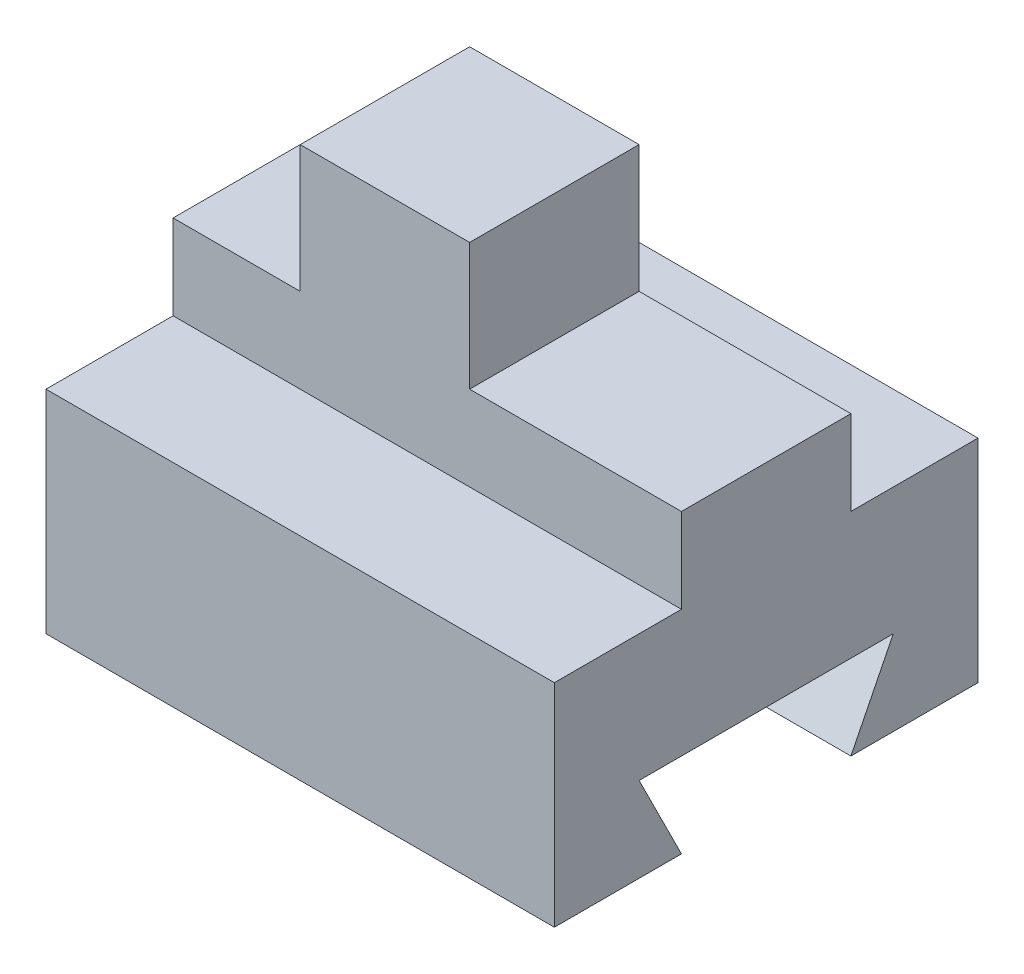
ISO-10303-21;
HEADER;
FILE_DESCRIPTION(('STEP AP214'),'2;1');
FILE_NAME('part.step','',(''),(''),'','','');
FILE_SCHEMA(('AUTOMOTIVE_DESIGN { 1 0 10303 214 1 1 1 1 }'));
ENDSEC;
DATA;
#1=APPLICATION_CONTEXT('core data for automotive mechanical design processes');
#2=APPLICATION_PROTOCOL_DEFINITION('international standard','automotive_design',2000,#1);
#3=PRODUCT_CONTEXT('',#1,'mechanical');
#4=PRODUCT('Part','Part','',(#3));
#5=PRODUCT_RELATED_PRODUCT_CATEGORY('part','',(#4));
#6=PRODUCT_DEFINITION_FORMATION('','',#4);
#7=PRODUCT_DEFINITION_CONTEXT('part definition',#1,'design');
#8=PRODUCT_DEFINITION('design','',#6,#7);
#9=PRODUCT_DEFINITION_SHAPE('','',#8);
#10=(LENGTH_UNIT() NAMED_UNIT(*) SI_UNIT(.MILLI.,.METRE.));
#11=(NAMED_UNIT(*) PLANE_ANGLE_UNIT() SI_UNIT($,.RADIAN.));
#12=(NAMED_UNIT(*) SI_UNIT($,.STERADIAN.) SOLID_ANGLE_UNIT());
#13=UNCERTAINTY_MEASURE_WITH_UNIT(LENGTH_MEASURE(1.E-05),#10,'distance_accuracy_value','');
#14=(GEOMETRIC_REPRESENTATION_CONTEXT(3) GLOBAL_UNCERTAINTY_ASSIGNED_CONTEXT((#13)) GLOBAL_UNIT_ASSIGNED_CONTEXT((#10,
#11,#12)) REPRESENTATION_CONTEXT('',''));
#15=CARTESIAN_POINT('',(0.,0.,0.));
#16=DIRECTION('',(0.,0.,1.));
#17=DIRECTION('',(1.,0.,0.));
#18=AXIS2_PLACEMENT_3D('',#15,#16,#17);
#19=CARTESIAN_POINT('',(30.,0.,25.));
#20=DIRECTION('',(0.,1.,0.));
#21=DIRECTION('',(0.,0.,1.));
#22=AXIS2_PLACEMENT_3D('',#19,#20,#21);
#23=PLANE('',#22);
#24=DIRECTION('',(1.,0.,0.));
#25=VECTOR('',#24,1.);
#26=CARTESIAN_POINT('',(-30.001,0.,-10.));
#27=LINE('',#26,#25);
#28=CARTESIAN_POINT('',(-30.,0.,-10.));
#29=VERTEX_POINT('',#28);
#30=CARTESIAN_POINT('',(30.,0.,-10.));
#31=VERTEX_POINT('',#30);
#32=EDGE_CURVE('E154',#29,#31,#27,.T.);
#33=ORIENTED_EDGE('',*,*,#32,.F.);
#34=DIRECTION('',(0.,0.,-1.));
#35=VECTOR('',#34,1.);
#36=CARTESIAN_POINT('',(-30.,0.,25.));
#37=LINE('',#36,#35);
#38=CARTESIAN_POINT('',(-30.,0.,-25.));
#39=VERTEX_POINT('',#38);
#40=EDGE_CURVE('E169',#29,#39,#37,.T.);
#41=ORIENTED_EDGE('',*,*,#40,.T.);
#42=DIRECTION('',(-1.,0.,0.));
#43=VECTOR('',#42,1.);
#44=CARTESIAN_POINT('',(30.,0.,-25.));
#45=LINE('',#44,#43);
#46=CARTESIAN_POINT('',(30.,0.,-25.));
#47=VERTEX_POINT('',#46);
#48=EDGE_CURVE('E50',#47,#39,#45,.T.);
#49=ORIENTED_EDGE('',*,*,#48,.F.);
#50=DIRECTION('',(0.,0.,-1.));
#51=VECTOR('',#50,1.);
#52=CARTESIAN_POINT('',(30.,0.,25.));
#53=LINE('',#52,#51);
#54=EDGE_CURVE('E168',#31,#47,#53,.T.);
#55=ORIENTED_EDGE('',*,*,#54,.F.);
#56=EDGE_LOOP('',(#33,#41,#49,#55));
#57=FACE_BOUND('',#56,.T.);
#58=ADVANCED_FACE('F39',(#57),#23,.F.);
#59=CARTESIAN_POINT('',(-30.,0.,0.));
#60=DIRECTION('',(1.,0.,0.));
#61=DIRECTION('',(0.,0.,-1.));
#62=AXIS2_PLACEMENT_3D('',#59,#60,#61);
#63=PLANE('',#62);
#64=DIRECTION('',(0.,0.894427190999916,0.447213595499958));
#65=VECTOR('',#64,1.);
#66=CARTESIAN_POINT('',(-30.,0.,10.));
#67=LINE('',#66,#65);
#68=CARTESIAN_POINT('',(-30.,0.,10.));
#69=VERTEX_POINT('',#68);
#70=CARTESIAN_POINT('',(-30.,10.,15.));
#71=VERTEX_POINT('',#70);
#72=EDGE_CURVE('E53',#69,#71,#67,.T.);
#73=ORIENTED_EDGE('',*,*,#72,.F.);
#74=CARTESIAN_POINT('',(-30.,0.,25.));
#75=VERTEX_POINT('',#74);
#76=EDGE_CURVE('E177',#75,#69,#37,.T.);
#77=ORIENTED_EDGE('',*,*,#76,.F.);
#78=DIRECTION('',(0.,-1.,0.));
#79=VECTOR('',#78,1.);
#80=CARTESIAN_POINT('',(-30.,25.,25.));
#81=LINE('',#80,#79);
#82=CARTESIAN_POINT('',(-30.,25.,25.));
#83=VERTEX_POINT('',#82);
#84=EDGE_CURVE('E179',#83,#75,#81,.T.);
#85=ORIENTED_EDGE('',*,*,#84,.F.);
#86=DIRECTION('',(0.,0.,1.));
#87=VECTOR('',#86,1.);
#88=CARTESIAN_POINT('',(-30.,25.,10.));
#89=LINE('',#88,#87);
#90=CARTESIAN_POINT('',(-30.,25.,10.));
#91=VERTEX_POINT('',#90);
#92=EDGE_CURVE('E193',#91,#83,#89,.T.);
#93=ORIENTED_EDGE('',*,*,#92,.F.);
#94=DIRECTION('',(0.,-1.,0.));
#95=VECTOR('',#94,1.);
#96=CARTESIAN_POINT('',(-30.,50.,10.));
#97=LINE('',#96,#95);
#98=CARTESIAN_POINT('',(-30.,35.,10.));
#99=VERTEX_POINT('',#98);
#100=EDGE_CURVE('E192',#99,#91,#97,.T.);
#101=ORIENTED_EDGE('',*,*,#100,.F.);
#102=DIRECTION('',(0.,0.,1.));
#103=VECTOR('',#102,1.);
#104=CARTESIAN_POINT('',(-30.,35.,-25.001));
#105=LINE('',#104,#103);
#106=CARTESIAN_POINT('',(-30.,35.,-10.));
#107=VERTEX_POINT('',#106);
#108=EDGE_CURVE('E264',#107,#99,#105,.T.);
#109=ORIENTED_EDGE('',*,*,#108,.F.);
#110=DIRECTION('',(0.,1.,0.));
#111=VECTOR('',#110,1.);
#112=CARTESIAN_POINT('',(-30.,25.,-10.));
#113=LINE('',#112,#111);
#114=CARTESIAN_POINT('',(-30.,25.,-10.));
#115=VERTEX_POINT('',#114);
#116=EDGE_CURVE('E188',#115,#107,#113,.T.);
#117=ORIENTED_EDGE('',*,*,#116,.F.);
#118=DIRECTION('',(0.,0.,1.));
#119=VECTOR('',#118,1.);
#120=CARTESIAN_POINT('',(-30.,25.,-25.));
#121=LINE('',#120,#119);
#122=CARTESIAN_POINT('',(-30.,25.,-25.));
#123=VERTEX_POINT('',#122);
#124=EDGE_CURVE('E190',#123,#115,#121,.T.);
#125=ORIENTED_EDGE('',*,*,#124,.F.);
#126=DIRECTION('',(0.,1.,0.));
#127=VECTOR('',#126,1.);
#128=CARTESIAN_POINT('',(-30.,0.,-25.));
#129=LINE('',#128,#127);
#130=EDGE_CURVE('E176',#39,#123,#129,.T.);
#131=ORIENTED_EDGE('',*,*,#130,.F.);
#132=ORIENTED_EDGE('',*,*,#40,.F.);
#133=DIRECTION('',(0.,-0.894427190999916,0.447213595499958));
#134=VECTOR('',#133,1.);
#135=CARTESIAN_POINT('',(-30.,10.,-15.));
#136=LINE('',#135,#134);
#137=CARTESIAN_POINT('',(-30.,10.,-15.));
#138=VERTEX_POINT('',#137);
#139=EDGE_CURVE('E151',#138,#29,#136,.T.);
#140=ORIENTED_EDGE('',*,*,#139,.F.);
#141=DIRECTION('',(0.,0.,-1.));
#142=VECTOR('',#141,1.);
#143=CARTESIAN_POINT('',(-30.,10.,15.));
#144=LINE('',#143,#142);
#145=EDGE_CURVE('E290',#71,#138,#144,.T.);
#146=ORIENTED_EDGE('',*,*,#145,.F.);
#147=EDGE_LOOP('',(#73,#77,#85,#93,#101,#109,#117,#125,#131,#132,#140,#146));
#148=FACE_BOUND('',#147,.T.);
#149=ADVANCED_FACE('F173',(#148),#63,.F.);
#150=CARTESIAN_POINT('',(30.,25.,-10.));
#151=DIRECTION('',(0.,0.,1.));
#152=DIRECTION('',(1.,0.,0.));
#153=AXIS2_PLACEMENT_3D('',#150,#151,#152);
#154=PLANE('',#153);
#155=DIRECTION('',(0.,-1.,0.));
#156=VECTOR('',#155,1.);
#157=CARTESIAN_POINT('',(-15.,0.,-10.));
#158=LINE('',#157,#156);
#159=CARTESIAN_POINT('',(-15.,50.,-10.));
#160=VERTEX_POINT('',#159);
#161=CARTESIAN_POINT('',(-15.,35.,-10.));
#162=VERTEX_POINT('',#161);
#163=EDGE_CURVE('E185',#160,#162,#158,.T.);
#164=ORIENTED_EDGE('',*,*,#163,.F.);
#165=DIRECTION('',(-1.,0.,0.));
#166=VECTOR('',#165,1.);
#167=CARTESIAN_POINT('',(30.,50.,-10.));
#168=LINE('',#167,#166);
#169=CARTESIAN_POINT('',(5.,50.,-10.));
#170=VERTEX_POINT('',#169);
#171=EDGE_CURVE('E210',#170,#160,#168,.T.);
#172=ORIENTED_EDGE('',*,*,#171,.F.);
#173=DIRECTION('',(0.,1.,0.));
#174=VECTOR('',#173,1.);
#175=CARTESIAN_POINT('',(5.00000000000001,0.,-10.));
#176=LINE('',#175,#174);
#177=CARTESIAN_POINT('',(5.,35.,-10.));
#178=VERTEX_POINT('',#177);
#179=EDGE_CURVE('E165',#178,#170,#176,.T.);
#180=ORIENTED_EDGE('',*,*,#179,.F.);
#181=DIRECTION('',(-1.,0.,0.));
#182=VECTOR('',#181,1.);
#183=CARTESIAN_POINT('',(0.,35.,-10.));
#184=LINE('',#183,#182);
#185=CARTESIAN_POINT('',(30.,35.,-10.));
#186=VERTEX_POINT('',#185);
#187=EDGE_CURVE('E249',#186,#178,#184,.T.);
#188=ORIENTED_EDGE('',*,*,#187,.F.);
#189=DIRECTION('',(0.,1.,0.));
#190=VECTOR('',#189,1.);
#191=CARTESIAN_POINT('',(30.,25.,-10.));
#192=LINE('',#191,#190);
#193=CARTESIAN_POINT('',(30.,25.,-10.));
#194=VERTEX_POINT('',#193);
#195=EDGE_CURVE('E223',#194,#186,#192,.T.);
#196=ORIENTED_EDGE('',*,*,#195,.F.);
#197=DIRECTION('',(-1.,0.,0.));
#198=VECTOR('',#197,1.);
#199=CARTESIAN_POINT('',(30.,25.,-10.));
#200=LINE('',#199,#198);
#201=EDGE_CURVE('E209',#194,#115,#200,.T.);
#202=ORIENTED_EDGE('',*,*,#201,.T.);
#203=ORIENTED_EDGE('',*,*,#116,.T.);
#204=DIRECTION('',(-1.,0.,0.));
#205=VECTOR('',#204,1.);
#206=CARTESIAN_POINT('',(0.,35.,-10.));
#207=LINE('',#206,#205);
#208=EDGE_CURVE('E253',#162,#107,#207,.T.);
#209=ORIENTED_EDGE('',*,*,#208,.F.);
#210=EDGE_LOOP('',(#164,#172,#180,#188,#196,#202,#203,#209));
#211=FACE_BOUND('',#210,.T.);
#212=ADVANCED_FACE('F307',(#211),#154,.F.);
#213=CARTESIAN_POINT('',(30.,50.,-10.));
#214=DIRECTION('',(0.,-1.,0.));
#215=DIRECTION('',(0.,0.,-1.));
#216=AXIS2_PLACEMENT_3D('',#213,#214,#215);
#217=PLANE('',#216);
#218=ORIENTED_EDGE('',*,*,#171,.T.);
#219=DIRECTION('',(0.,0.,1.));
#220=VECTOR('',#219,1.);
#221=CARTESIAN_POINT('',(-15.,50.,-25.001));
#222=LINE('',#221,#220);
#223=CARTESIAN_POINT('',(-15.,50.,10.));
#224=VERTEX_POINT('',#223);
#225=EDGE_CURVE('E268',#160,#224,#222,.T.);
#226=ORIENTED_EDGE('',*,*,#225,.T.);
#227=DIRECTION('',(-1.,0.,0.));
#228=VECTOR('',#227,1.);
#229=CARTESIAN_POINT('',(30.,50.,10.));
#230=LINE('',#229,#228);
#231=CARTESIAN_POINT('',(5.,50.,10.));
#232=VERTEX_POINT('',#231);
#233=EDGE_CURVE('E204',#232,#224,#230,.T.);
#234=ORIENTED_EDGE('',*,*,#233,.F.);
#235=DIRECTION('',(0.,0.,1.));
#236=VECTOR('',#235,1.);
#237=CARTESIAN_POINT('',(5.,50.,-25.001));
#238=LINE('',#237,#236);
#239=EDGE_CURVE('E252',#170,#232,#238,.T.);
#240=ORIENTED_EDGE('',*,*,#239,.F.);
#241=EDGE_LOOP('',(#218,#226,#234,#240));
#242=FACE_BOUND('',#241,.T.);
#243=ADVANCED_FACE('F325',(#242),#217,.F.);
#244=CARTESIAN_POINT('',(30.,50.,10.));
#245=DIRECTION('',(0.,0.,-1.));
#246=DIRECTION('',(-1.,0.,0.));
#247=AXIS2_PLACEMENT_3D('',#244,#245,#246);
#248=PLANE('',#247);
#249=DIRECTION('',(1.,0.,0.));
#250=VECTOR('',#249,1.);
#251=CARTESIAN_POINT('',(0.,35.,10.));
#252=LINE('',#251,#250);
#253=CARTESIAN_POINT('',(-15.,35.,10.));
#254=VERTEX_POINT('',#253);
#255=EDGE_CURVE('E273',#99,#254,#252,.T.);
#256=ORIENTED_EDGE('',*,*,#255,.F.);
#257=ORIENTED_EDGE('',*,*,#100,.T.);
#258=DIRECTION('',(-1.,0.,0.));
#259=VECTOR('',#258,1.);
#260=CARTESIAN_POINT('',(30.,25.,10.));
#261=LINE('',#260,#259);
#262=CARTESIAN_POINT('',(30.,25.,10.));
#263=VERTEX_POINT('',#262);
#264=EDGE_CURVE('E199',#263,#91,#261,.T.);
#265=ORIENTED_EDGE('',*,*,#264,.F.);
#266=DIRECTION('',(0.,-1.,0.));
#267=VECTOR('',#266,1.);
#268=CARTESIAN_POINT('',(30.,50.,10.));
#269=LINE('',#268,#267);
#270=CARTESIAN_POINT('',(30.,35.,10.));
#271=VERTEX_POINT('',#270);
#272=EDGE_CURVE('E234',#271,#263,#269,.T.);
#273=ORIENTED_EDGE('',*,*,#272,.F.);
#274=DIRECTION('',(1.,0.,0.));
#275=VECTOR('',#274,1.);
#276=CARTESIAN_POINT('',(0.,35.,10.));
#277=LINE('',#276,#275);
#278=CARTESIAN_POINT('',(5.,35.,10.));
#279=VERTEX_POINT('',#278);
#280=EDGE_CURVE('E65',#279,#271,#277,.T.);
#281=ORIENTED_EDGE('',*,*,#280,.F.);
#282=DIRECTION('',(0.,-1.,0.));
#283=VECTOR('',#282,1.);
#284=CARTESIAN_POINT('',(5.00000000000001,0.,10.));
#285=LINE('',#284,#283);
#286=EDGE_CURVE('E259',#232,#279,#285,.T.);
#287=ORIENTED_EDGE('',*,*,#286,.F.);
#288=ORIENTED_EDGE('',*,*,#233,.T.);
#289=DIRECTION('',(0.,1.,0.));
#290=VECTOR('',#289,1.);
#291=CARTESIAN_POINT('',(-15.,0.,10.));
#292=LINE('',#291,#290);
#293=EDGE_CURVE('E267',#254,#224,#292,.T.);
#294=ORIENTED_EDGE('',*,*,#293,.F.);
#295=EDGE_LOOP('',(#256,#257,#265,#273,#281,#287,#288,#294));
#296=FACE_BOUND('',#295,.T.);
#297=ADVANCED_FACE('F299',(#296),#248,.F.);
#298=CARTESIAN_POINT('',(30.,0.,0.));
#299=DIRECTION('',(1.,0.,0.));
#300=DIRECTION('',(0.,0.,-1.));
#301=AXIS2_PLACEMENT_3D('',#298,#299,#300);
#302=PLANE('',#301);
#303=DIRECTION('',(0.,0.894427190999916,-0.447213595499958));
#304=VECTOR('',#303,1.);
#305=CARTESIAN_POINT('',(30.,10.,-15.));
#306=LINE('',#305,#304);
#307=CARTESIAN_POINT('',(30.,10.,-15.));
#308=VERTEX_POINT('',#307);
#309=EDGE_CURVE('E287',#31,#308,#306,.T.);
#310=ORIENTED_EDGE('',*,*,#309,.F.);
#311=ORIENTED_EDGE('',*,*,#54,.T.);
#312=DIRECTION('',(0.,1.,0.));
#313=VECTOR('',#312,1.);
#314=CARTESIAN_POINT('',(30.,0.,-25.));
#315=LINE('',#314,#313);
#316=CARTESIAN_POINT('',(30.,25.,-25.));
#317=VERTEX_POINT('',#316);
#318=EDGE_CURVE('E218',#47,#317,#315,.T.);
#319=ORIENTED_EDGE('',*,*,#318,.T.);
#320=DIRECTION('',(0.,0.,1.));
#321=VECTOR('',#320,1.);
#322=CARTESIAN_POINT('',(30.,25.,-25.));
#323=LINE('',#322,#321);
#324=EDGE_CURVE('E225',#317,#194,#323,.T.);
#325=ORIENTED_EDGE('',*,*,#324,.T.);
#326=ORIENTED_EDGE('',*,*,#195,.T.);
#327=DIRECTION('',(0.,0.,1.));
#328=VECTOR('',#327,1.);
#329=CARTESIAN_POINT('',(30.,35.,-25.001));
#330=LINE('',#329,#328);
#331=EDGE_CURVE('E254',#186,#271,#330,.T.);
#332=ORIENTED_EDGE('',*,*,#331,.T.);
#333=ORIENTED_EDGE('',*,*,#272,.T.);
#334=DIRECTION('',(0.,0.,1.));
#335=VECTOR('',#334,1.);
#336=CARTESIAN_POINT('',(30.,25.,10.));
#337=LINE('',#336,#335);
#338=CARTESIAN_POINT('',(30.,25.,25.));
#339=VERTEX_POINT('',#338);
#340=EDGE_CURVE('E203',#263,#339,#337,.T.);
#341=ORIENTED_EDGE('',*,*,#340,.T.);
#342=DIRECTION('',(0.,-1.,0.));
#343=VECTOR('',#342,1.);
#344=CARTESIAN_POINT('',(30.,25.,25.));
#345=LINE('',#344,#343);
#346=CARTESIAN_POINT('',(30.,0.,25.));
#347=VERTEX_POINT('',#346);
#348=EDGE_CURVE('E198',#339,#347,#345,.T.);
#349=ORIENTED_EDGE('',*,*,#348,.T.);
#350=CARTESIAN_POINT('',(30.,0.,10.));
#351=VERTEX_POINT('',#350);
#352=EDGE_CURVE('E224',#347,#351,#53,.T.);
#353=ORIENTED_EDGE('',*,*,#352,.T.);
#354=DIRECTION('',(0.,-0.894427190999916,-0.447213595499958));
#355=VECTOR('',#354,1.);
#356=CARTESIAN_POINT('',(30.,0.,10.));
#357=LINE('',#356,#355);
#358=CARTESIAN_POINT('',(30.,10.,15.));
#359=VERTEX_POINT('',#358);
#360=EDGE_CURVE('E171',#359,#351,#357,.T.);
#361=ORIENTED_EDGE('',*,*,#360,.F.);
#362=DIRECTION('',(0.,0.,1.));
#363=VECTOR('',#362,1.);
#364=CARTESIAN_POINT('',(30.,10.,15.));
#365=LINE('',#364,#363);
#366=EDGE_CURVE('E283',#308,#359,#365,.T.);
#367=ORIENTED_EDGE('',*,*,#366,.F.);
#368=EDGE_LOOP('',(#310,#311,#319,#325,#326,#332,#333,#341,#349,#353,#361,#367));
#369=FACE_BOUND('',#368,.T.);
#370=ADVANCED_FACE('F240',(#369),#302,.T.);
#371=CARTESIAN_POINT('',(30.,25.,25.));
#372=DIRECTION('',(0.,0.,-1.));
#373=DIRECTION('',(0.,1.,0.));
#374=AXIS2_PLACEMENT_3D('',#371,#372,#373);
#375=PLANE('',#374);
#376=ORIENTED_EDGE('',*,*,#84,.T.);
#377=DIRECTION('',(-1.,0.,0.));
#378=VECTOR('',#377,1.);
#379=CARTESIAN_POINT('',(30.,0.,25.));
#380=LINE('',#379,#378);
#381=EDGE_CURVE('E11',#347,#75,#380,.T.);
#382=ORIENTED_EDGE('',*,*,#381,.F.);
#383=ORIENTED_EDGE('',*,*,#348,.F.);
#384=DIRECTION('',(-1.,0.,0.));
#385=VECTOR('',#384,1.);
#386=CARTESIAN_POINT('',(30.,25.,25.));
#387=LINE('',#386,#385);
#388=EDGE_CURVE('E197',#339,#83,#387,.T.);
#389=ORIENTED_EDGE('',*,*,#388,.T.);
#390=EDGE_LOOP('',(#376,#382,#383,#389));
#391=FACE_BOUND('',#390,.T.);
#392=ADVANCED_FACE('F41',(#391),#375,.F.);
#393=ORIENTED_EDGE('',*,*,#76,.T.);
#394=DIRECTION('',(1.,0.,0.));
#395=VECTOR('',#394,1.);
#396=CARTESIAN_POINT('',(-30.001,0.,10.));
#397=LINE('',#396,#395);
#398=EDGE_CURVE('E162',#69,#351,#397,.T.);
#399=ORIENTED_EDGE('',*,*,#398,.T.);
#400=ORIENTED_EDGE('',*,*,#352,.F.);
#401=ORIENTED_EDGE('',*,*,#381,.T.);
#402=EDGE_LOOP('',(#393,#399,#400,#401));
#403=FACE_BOUND('',#402,.T.);
#404=ADVANCED_FACE('F294',(#403),#23,.F.);
#405=CARTESIAN_POINT('',(30.,0.,-25.));
#406=DIRECTION('',(0.,0.,1.));
#407=DIRECTION('',(0.,-1.,0.));
#408=AXIS2_PLACEMENT_3D('',#405,#406,#407);
#409=PLANE('',#408);
#410=ORIENTED_EDGE('',*,*,#130,.T.);
#411=DIRECTION('',(-1.,0.,0.));
#412=VECTOR('',#411,1.);
#413=CARTESIAN_POINT('',(30.,25.,-25.));
#414=LINE('',#413,#412);
#415=EDGE_CURVE('E213',#317,#123,#414,.T.);
#416=ORIENTED_EDGE('',*,*,#415,.F.);
#417=ORIENTED_EDGE('',*,*,#318,.F.);
#418=ORIENTED_EDGE('',*,*,#48,.T.);
#419=EDGE_LOOP('',(#410,#416,#417,#418));
#420=FACE_BOUND('',#419,.T.);
#421=ADVANCED_FACE('F220',(#420),#409,.F.);
#422=CARTESIAN_POINT('',(30.,25.,-25.));
#423=DIRECTION('',(0.,-1.,0.));
#424=DIRECTION('',(0.,0.,-1.));
#425=AXIS2_PLACEMENT_3D('',#422,#423,#424);
#426=PLANE('',#425);
#427=ORIENTED_EDGE('',*,*,#124,.T.);
#428=ORIENTED_EDGE('',*,*,#201,.F.);
#429=ORIENTED_EDGE('',*,*,#324,.F.);
#430=ORIENTED_EDGE('',*,*,#415,.T.);
#431=EDGE_LOOP('',(#427,#428,#429,#430));
#432=FACE_BOUND('',#431,.T.);
#433=ADVANCED_FACE('F315',(#432),#426,.F.);
#434=CARTESIAN_POINT('',(30.,25.,10.));
#435=DIRECTION('',(0.,-1.,0.));
#436=DIRECTION('',(0.,0.,-1.));
#437=AXIS2_PLACEMENT_3D('',#434,#435,#436);
#438=PLANE('',#437);
#439=ORIENTED_EDGE('',*,*,#92,.T.);
#440=ORIENTED_EDGE('',*,*,#388,.F.);
#441=ORIENTED_EDGE('',*,*,#340,.F.);
#442=ORIENTED_EDGE('',*,*,#264,.T.);
#443=EDGE_LOOP('',(#439,#440,#441,#442));
#444=FACE_BOUND('',#443,.T.);
#445=ADVANCED_FACE('F242',(#444),#438,.F.);
#446=CARTESIAN_POINT('',(0.,35.,-25.001));
#447=DIRECTION('',(0.,-1.,0.));
#448=DIRECTION('',(1.,0.,0.));
#449=AXIS2_PLACEMENT_3D('',#446,#447,#448);
#450=PLANE('',#449);
#451=ORIENTED_EDGE('',*,*,#208,.T.);
#452=ORIENTED_EDGE('',*,*,#108,.T.);
#453=ORIENTED_EDGE('',*,*,#255,.T.);
#454=DIRECTION('',(0.,0.,1.));
#455=VECTOR('',#454,1.);
#456=CARTESIAN_POINT('',(-15.,35.,-25.001));
#457=LINE('',#456,#455);
#458=EDGE_CURVE('E266',#162,#254,#457,.T.);
#459=ORIENTED_EDGE('',*,*,#458,.F.);
#460=EDGE_LOOP('',(#451,#452,#453,#459));
#461=FACE_BOUND('',#460,.T.);
#462=ADVANCED_FACE('F304',(#461),#450,.F.);
#463=CARTESIAN_POINT('',(-15.,0.,-25.001));
#464=DIRECTION('',(1.,0.,0.));
#465=DIRECTION('',(0.,0.,-1.));
#466=AXIS2_PLACEMENT_3D('',#463,#464,#465);
#467=PLANE('',#466);
#468=ORIENTED_EDGE('',*,*,#163,.T.);
#469=ORIENTED_EDGE('',*,*,#458,.T.);
#470=ORIENTED_EDGE('',*,*,#293,.T.);
#471=ORIENTED_EDGE('',*,*,#225,.F.);
#472=EDGE_LOOP('',(#468,#469,#470,#471));
#473=FACE_BOUND('',#472,.T.);
#474=ADVANCED_FACE('F322',(#473),#467,.F.);
#475=CARTESIAN_POINT('',(5.00000000000001,0.,-25.001));
#476=DIRECTION('',(-1.,0.,0.));
#477=DIRECTION('',(0.,-1.,0.));
#478=AXIS2_PLACEMENT_3D('',#475,#476,#477);
#479=PLANE('',#478);
#480=ORIENTED_EDGE('',*,*,#179,.T.);
#481=ORIENTED_EDGE('',*,*,#239,.T.);
#482=ORIENTED_EDGE('',*,*,#286,.T.);
#483=DIRECTION('',(0.,0.,1.));
#484=VECTOR('',#483,1.);
#485=CARTESIAN_POINT('',(5.,35.,-25.001));
#486=LINE('',#485,#484);
#487=EDGE_CURVE('E251',#178,#279,#486,.T.);
#488=ORIENTED_EDGE('',*,*,#487,.F.);
#489=EDGE_LOOP('',(#480,#481,#482,#488));
#490=FACE_BOUND('',#489,.T.);
#491=ADVANCED_FACE('F318',(#490),#479,.F.);
#492=CARTESIAN_POINT('',(0.,35.,-25.001));
#493=DIRECTION('',(0.,-1.,0.));
#494=DIRECTION('',(0.,0.,-1.));
#495=AXIS2_PLACEMENT_3D('',#492,#493,#494);
#496=PLANE('',#495);
#497=ORIENTED_EDGE('',*,*,#187,.T.);
#498=ORIENTED_EDGE('',*,*,#487,.T.);
#499=ORIENTED_EDGE('',*,*,#280,.T.);
#500=ORIENTED_EDGE('',*,*,#331,.F.);
#501=EDGE_LOOP('',(#497,#498,#499,#500));
#502=FACE_BOUND('',#501,.T.);
#503=ADVANCED_FACE('F312',(#502),#496,.F.);
#504=CARTESIAN_POINT('',(-30.001,0.,10.));
#505=DIRECTION('',(0.,-0.447213595499958,0.894427190999916));
#506=DIRECTION('',(0.,-0.894427190999916,-0.447213595499958));
#507=AXIS2_PLACEMENT_3D('',#504,#505,#506);
#508=PLANE('',#507);
#509=ORIENTED_EDGE('',*,*,#72,.T.);
#510=DIRECTION('',(1.,0.,0.));
#511=VECTOR('',#510,1.);
#512=CARTESIAN_POINT('',(-30.001,10.,15.));
#513=LINE('',#512,#511);
#514=EDGE_CURVE('E276',#71,#359,#513,.T.);
#515=ORIENTED_EDGE('',*,*,#514,.T.);
#516=ORIENTED_EDGE('',*,*,#360,.T.);
#517=ORIENTED_EDGE('',*,*,#398,.F.);
#518=EDGE_LOOP('',(#509,#515,#516,#517));
#519=FACE_BOUND('',#518,.T.);
#520=ADVANCED_FACE('F412',(#519),#508,.F.);
#521=CARTESIAN_POINT('',(-30.001,10.,15.));
#522=DIRECTION('',(0.,1.,0.));
#523=DIRECTION('',(0.,0.,1.));
#524=AXIS2_PLACEMENT_3D('',#521,#522,#523);
#525=PLANE('',#524);
#526=ORIENTED_EDGE('',*,*,#145,.T.);
#527=DIRECTION('',(1.,0.,0.));
#528=VECTOR('',#527,1.);
#529=CARTESIAN_POINT('',(-30.001,10.,-15.));
#530=LINE('',#529,#528);
#531=EDGE_CURVE('E160',#138,#308,#530,.T.);
#532=ORIENTED_EDGE('',*,*,#531,.T.);
#533=ORIENTED_EDGE('',*,*,#366,.T.);
#534=ORIENTED_EDGE('',*,*,#514,.F.);
#535=EDGE_LOOP('',(#526,#532,#533,#534));
#536=FACE_BOUND('',#535,.T.);
#537=ADVANCED_FACE('F295',(#536),#525,.F.);
#538=CARTESIAN_POINT('',(-30.001,10.,-15.));
#539=DIRECTION('',(0.,-0.447213595499958,-0.894427190999916));
#540=DIRECTION('',(0.,0.894427190999916,-0.447213595499958));
#541=AXIS2_PLACEMENT_3D('',#538,#539,#540);
#542=PLANE('',#541);
#543=ORIENTED_EDGE('',*,*,#139,.T.);
#544=ORIENTED_EDGE('',*,*,#32,.T.);
#545=ORIENTED_EDGE('',*,*,#309,.T.);
#546=ORIENTED_EDGE('',*,*,#531,.F.);
#547=EDGE_LOOP('',(#543,#544,#545,#546));
#548=FACE_BOUND('',#547,.T.);
#549=ADVANCED_FACE('F153',(#548),#542,.F.);
#550=CLOSED_SHELL('',(#58,#149,#212,#243,#297,#370,#392,#404,#421,#433,#445,#462,#474,#491,#503,
#520,#537,#549));
#551=MANIFOLD_SOLID_BREP('B2',#550);
#552=ADVANCED_BREP_SHAPE_REPRESENTATION('',(#18,#551),#14);
#553=SHAPE_DEFINITION_REPRESENTATION(#9,#552);
ENDSEC;
END-ISO-10303-21;
